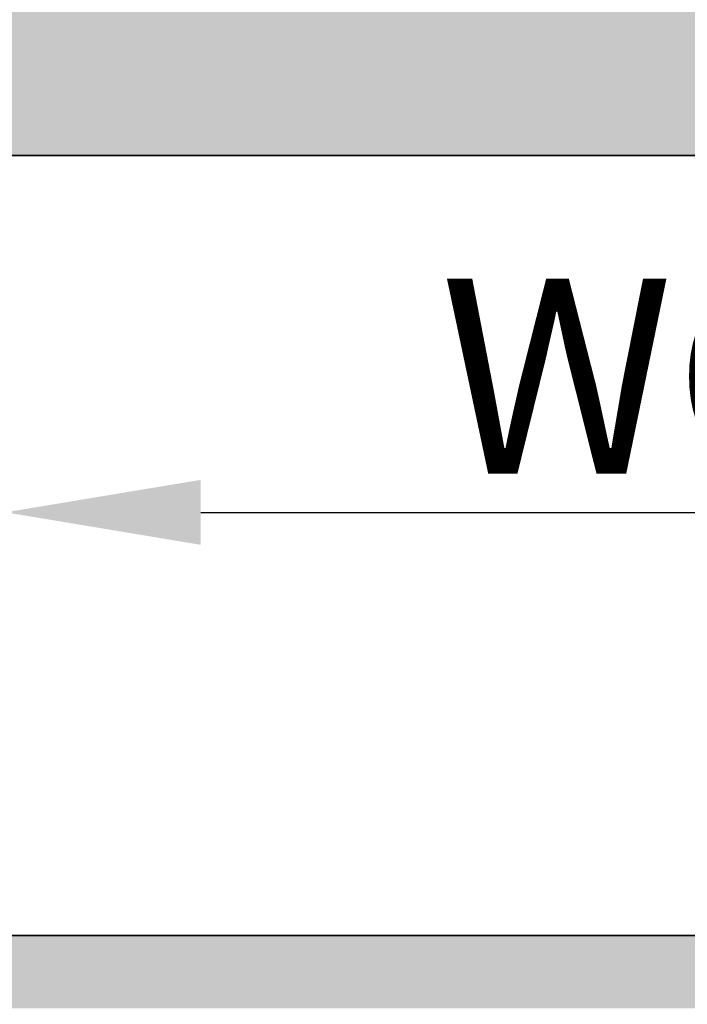
# Model space of a CAD drawing. Units: inches. Extents: x 2083 to 3317, y 1141 to 2115.
# Tile 17 of 256: x 2255 to 2296, y 1417 to 1477. Entities that reach past the tile are written whole.
import ezdxf

# ---------------------------------------------------------------- set-up
doc = ezdxf.new("R2010")
doc.units = ezdxf.units.IN
doc.layers.add('A-ANNO-DIMS', color=2, linetype='Continuous', lineweight=18)
doc.layers.add('A-WALL', color=7, linetype='Continuous', lineweight=35)
doc.layers.add('A-WALL-PATT', color=251, linetype='Continuous', lineweight=13, true_color=0x636466)
doc.styles.get("Standard").update_dxf_attribs({"font": 'arial.ttf'})
doc.dimstyles.new('ISO-25', dxfattribs={"dimtxt": 12, "dimasz": 12, "dimexe": 1.25, "dimexo": 0.625, "dimtad": 1, "dimlunit": 3, "dimtxsty": 'Standard', "dimcen": 2.5, "dimadec": 0, "dimazin": 0, "dimtfac": 1, "dimtmove": 0, "dimatfit": 3, "dimfxl": 1, "dimarcsym": 0})

# ---------------------------------------------------------------- blocks, each defined once
blk = doc.blocks.new('*D22')
at = {"layer": 'A-ANNO-DIMS', "color": 0, "lineweight": -2, "transparency": 16777216}
for p, q in [((2235.96, 1362.739), (2235.96, 1376.309)), ((2322.26, 1362.739), (2322.26, 1376.309)), ((2235.96, 1375.059), (2083.007, 1375.059)), ((2310.26, 1375.059), (2247.96, 1375.059))]:
    blk.add_line(p, q, dxfattribs=at)
at = {"layer": 'A-ANNO-DIMS', "color": 0, "transparency": 16777216}
for points in [[(2247.96, 1377.059), (2247.96, 1373.059), (2235.96, 1375.059)], [(2310.26, 1377.059), (2310.26, 1373.059), (2322.26, 1375.059)]]:
    blk.add_solid(points, dxfattribs=at)
at = {"layer": 'Defpoints', "color": 0, "transparency": 16777216}
for p in [(2235.96, 1375.059), (2235.96, 1362.114), (2322.26, 1362.114)]:
    blk.add_point(p, dxfattribs=at)
at = {"layer": 'A-ANNO-DIMS', "color": 0, "transparency": 16777216, "insert": (2153.483, 1381.889), "char_height": 12, "attachment_point": 5}
blk.add_mtext('BED 7\'-2 1/2" TYP.', dxfattribs=at)
blk = doc.blocks.new('*D30')
at = {"layer": 'A-ANNO-DIMS', "color": 0, "lineweight": -2, "transparency": 16777216}
for p, q in [((2240.018, 1445.274), (2240.018, 1448.046)), ((2254.329, 1445.274), (2254.329, 1448.046)), ((2228.018, 1446.796), (2216.018, 1446.796)), ((2240.018, 1446.796), (2254.329, 1446.796)), ((2266.329, 1446.796), (2413.765, 1446.796))]:
    blk.add_line(p, q, dxfattribs=at)
at = {"layer": 'A-ANNO-DIMS', "color": 0, "transparency": 16777216}
for points in [[(2228.018, 1448.796), (2228.018, 1444.796), (2240.018, 1446.796)], [(2266.329, 1448.796), (2266.329, 1444.796), (2254.329, 1446.796)]]:
    blk.add_solid(points, dxfattribs=at)
at = {"layer": 'Defpoints', "color": 0, "transparency": 16777216}
for p in [(2254.329, 1446.796), (2240.018, 1444.649), (2254.329, 1444.649)]:
    blk.add_point(p, dxfattribs=at)
at = {"layer": 'A-ANNO-DIMS', "color": 0, "transparency": 16777216, "insert": (2346.047, 1453.625), "char_height": 12, "attachment_point": 5}
blk.add_mtext('WC 1\'-2 1/2" TYP.', dxfattribs=at)
blk = doc.blocks.new('*D62')
at = {"layer": 'A-ANNO-DIMS', "color": 0, "lineweight": -2, "transparency": 16777216}
for p, q in [((2235.96, 1469.386), (2235.96, 1522.361)), ((2379.96, 1469.386), (2379.96, 1522.361)), ((2247.96, 1521.111), (2367.96, 1521.111))]:
    blk.add_line(p, q, dxfattribs=at)
at = {"layer": 'A-ANNO-DIMS', "color": 0, "transparency": 16777216}
for points in [[(2247.96, 1523.111), (2247.96, 1519.111), (2235.96, 1521.111)], [(2367.96, 1523.111), (2367.96, 1519.111), (2379.96, 1521.111)]]:
    blk.add_solid(points, dxfattribs=at)
at = {"layer": 'Defpoints', "color": 0, "transparency": 16777216}
for p in [(2379.96, 1521.111), (2235.96, 1468.761), (2379.96, 1468.761)]:
    blk.add_point(p, dxfattribs=at)
at = {"layer": 'A-ANNO-DIMS', "color": 0, "transparency": 16777216, "insert": (2307.96, 1527.863), "char_height": 12, "attachment_point": 5}
blk.add_mtext('12\'-0"', dxfattribs=at)

msp = doc.modelspace()

# ---------------------------------------------------------------- hatches: boundary and pattern name
at = {"layer": 'A-WALL-PATT'}
h = msp.add_hatch(color=256, dxfattribs=at)
h.dxf.hatch_style = 1
h.paths.add_polyline_path([(3126.96, 2020.761), (2748.96, 2020.761), (2604.96, 2020.761), (2226.96, 2020.761), (2226.96, 1702.761), (2466.96, 1702.761), (2466.96, 1582.761), (2418.96, 1582.761), (2418.96, 1477.761), (2226.96, 1477.761), (2226.96, 1263.261), (2544.96, 1263.261), (2544.96, 1411.761), (2604.96, 1411.761), (2685.96, 1411.761), (2685.96, 1420.761), (2604.96, 1420.761), (2604.96, 1573.761), (2604.96, 1702.761), (2604.96, 2011.761), (2748.96, 2011.761), (2748.96, 1702.761), (2862.96, 1702.761), (2862.96, 1621.761), (2871.96, 1621.761), (2871.96, 1702.761), (2883.96, 1702.761), (2883.96, 1706.939, -0.026459), (2883.96, 1711.761), (2757.96, 1711.761), (2757.96, 1807.761), (2787.96, 1807.761), (2787.96, 1812.261), (2757.96, 1812.261), (2757.96, 2011.761), (2877.96, 2011.761), (2877.96, 1812.261), (2847.96, 1812.261), (2847.96, 1807.761), (2889.836, 1807.761), (2889.836, 1812.261), (2882.46, 1812.261), (2882.46, 2011.761), (3117.96, 2011.761), (3117.96, 1812.261), (2937.836, 1812.261), (2937.836, 1807.761), (2995.71, 1807.761), (2995.71, 1796.118), (3000.21, 1796.118), (3000.21, 1807.761), (3117.96, 1807.761), (3117.96, 1711.761), (3000.21, 1711.761), (3000.21, 1760.118), (2998.573, 1760.118, -0.020711), (2995.71, 1760.118), (2995.71, 1711.761), (2931.96, 1711.761), (2931.96, 1702.761), (3126.96, 1702.761)])
h.paths.add_polyline_path([(2471.46, 2011.761), (2471.46, 1810.011), (2462.717, 1810.011), (2462.717, 1805.511), (2505.96, 1805.511), (2505.96, 1810.011), (2475.96, 1810.011), (2475.96, 2011.761), (2595.96, 2011.761), (2595.96, 1810.011), (2565.96, 1810.011), (2565.96, 1805.511), (2595.96, 1805.511), (2595.96, 1711.761), (2235.96, 1711.761), (2235.96, 1805.511), (2353.71, 1805.511), (2353.71, 1796.054), (2358.21, 1796.054), (2358.21, 1805.511), (2414.717, 1805.511), (2414.717, 1810.011), (2235.96, 1810.011), (2235.96, 2011.761)], flags=16)
h.paths.add_polyline_path([(2270.205, 1994.61), (2270.205, 1970.61), (2246.205, 1970.61), (2246.205, 1994.61)], flags=0)
edge = h.paths.add_edge_path(flags=0)
edge.add_ellipse((2332.027, 1899.798), major_axis=(-3.043, 3.043), ratio=0.168252, start_angle=-161.33217, end_angle=-156.30711, ccw=False)
edge.add_ellipse((2333.082, 1898.744), major_axis=(-1.055, 1.055), ratio=0.453532, start_angle=-123.37102, end_angle=-94.15911)
edge = h.paths.add_edge_path(flags=0)
edge.add_ellipse((2332.027, 1968.876), major_axis=(3.043, 3.043), ratio=0.168252, start_angle=18.66783, end_angle=23.69289)
edge.add_spline(control_points=[(2332.926, 1970.691), (2332.227, 1970.336), (2330.894, 1969.659), (2328.413, 1970.932), (2327.204, 1967.749), (2324.71, 1969.956), (2322.533, 1967.012), (2320.013, 1971.296), (2317.68, 1968.158), (2316.041, 1967.102), (2315.427, 1966.81)], knot_values=[0, 0, 0, 0, 2.267059, 4.324559, 6.685584, 8.878641, 11.121502, 14.300359, 17.755284, 19.732645, 19.732645, 19.732645, 19.732645], degree=3, periodic=0)
edge.add_ellipse((2332.027, 1968.876), major_axis=(3.043, 3.043), ratio=0.168252, start_angle=18.66783, end_angle=23.69289, ccw=False)
edge.add_ellipse((2333.082, 1969.931), major_axis=(1.055, 1.055), ratio=0.453532, start_angle=56.62898, end_angle=85.84089, ccw=False)
edge = h.paths.add_edge_path(flags=0)
edge.add_spline(control_points=[(2296.428, 1967.988), (2293.628, 1965.336), (2287.704, 1959.727), (2299.744, 1949.996), (2294.533, 1935.669), (2290.573, 1920.604), (2293.394, 1909.974), (2296.185, 1904.967)], knot_values=[0.099185, 0.099185, 0.099185, 0.099185, 0.345301, 0.619822, 0.982653, 1.386093, 1.810555, 1.810555, 1.810555, 1.810555], degree=3, periodic=0)
edge.add_spline(control_points=[(2296.185, 1904.967), (2297.384, 1902.619), (2298.001, 1901.949), (2298.553, 1901.468)], knot_values=[0.006246, 0.006246, 0.006246, 0.006246, 0.055476, 0.055476, 0.055476, 0.055476], degree=3, periodic=0)
edge.add_spline(control_points=[(2298.553, 1901.468), (2297.259, 1900.923), (2295.225, 1900.232), (2293.06, 1900.614), (2292.101, 1900.788), (2292.09, 1900.791)], knot_values=[0.312835, 0.312835, 0.312835, 0.312835, 0.40178, 0.474987, 0.475903, 0.475903, 0.475903, 0.475903], degree=3, periodic=0)
edge.add_arc((2292.794, 1904.664), 3.937, 215.4209, 259.69818, ccw=False)
edge.add_spline(control_points=[(2289.585, 1902.382), (2289.477, 1902.535), (2289.368, 1902.688), (2289.261, 1902.841)], knot_values=[0.102872, 0.102872, 0.102872, 0.102872, 0.116896, 0.116896, 0.116896, 0.116896], degree=3, periodic=0)
edge.add_spline(control_points=[(2289.261, 1902.841), (2288.687, 1902.55), (2287.64, 1902.02), (2285.881, 1901.874), (2283.853, 1901.504), (2281.72, 1899.711), (2278.467, 1899.493), (2276.157, 1901.883), (2272.259, 1899.804), (2267.778, 1901.843), (2262.244, 1900.184), (2257.415, 1901.782), (2254.318, 1900.726), (2253.178, 1900.337)], knot_values=[0, 0, 0, 0, 1.907977, 3.477176, 5.261074, 7.972851, 11.680248, 13.717921, 16.939592, 22.789562, 27.502503, 33.595215, 37.145618, 37.145618, 37.145618, 37.145618], degree=3, periodic=0)
edge.add_line((2253.178, 1900.337), (2250.244, 1902.841))
edge.add_line((2250.244, 1902.841), (2250.244, 1965.833))
edge.add_line((2250.244, 1965.833), (2253.178, 1968.337))
edge.add_spline(control_points=[(2253.178, 1968.337), (2254.318, 1967.948), (2257.415, 1966.892), (2262.244, 1968.49), (2267.778, 1966.831), (2271.527, 1968.537), (2273.876, 1967.828), (2274.207, 1967.728)], knot_values=[0, 0, 0, 0, 0.09018, 0.244935, 0.364644, 0.513233, 0.537855, 0.537855, 0.537855, 0.537855], degree=3, periodic=0)
edge.add_arc((2274.353, 1963.793), 3.937, 72.05113, 92.12795, ccw=False)
edge.add_arc((2281.297, 1985.23), 18.596, 252.05113, 288.56572)
edge.add_arc((2292.317, 1956.029), 12.646, 71.02679, 113.77822, ccw=False)
edge = h.paths.add_edge_path(flags=0)
edge.add_spline(control_points=[(2274.899, 1951.856), (2275.066, 1951.617), (2275.233, 1951.377), (2275.398, 1951.136)], knot_values=[1.409916, 1.409916, 1.409916, 1.409916, 1.43159, 1.43159, 1.43159, 1.43159], degree=3, periodic=0)
edge.add_spline(control_points=[(2275.398, 1951.136), (2275.792, 1950.562), (2276.179, 1949.984), (2276.546, 1949.397)], knot_values=[1.358238, 1.358238, 1.358238, 1.358238, 1.409916, 1.409916, 1.409916, 1.409916], degree=3, periodic=0)
edge.add_line((2276.546, 1949.397), (2277.437, 1947.862))
edge.add_spline(control_points=[(2277.437, 1947.862), (2276.304, 1945.673), (2274.64, 1942.427), (2274.632, 1938.094), (2272.799, 1930.852), (2274.356, 1943.897), (2275.948, 1947.923), (2276.546, 1949.397)], knot_values=[0.005632, 0.005632, 0.005632, 0.005632, 0.186014, 0.266002, 0.357087, 0.59639, 0.739732, 0.739732, 0.739732, 0.739732], degree=3, periodic=0)
edge.add_spline(control_points=[(2276.546, 1949.397), (2276.179, 1949.984), (2275.792, 1950.562), (2275.398, 1951.136)], knot_values=[1.358238, 1.358238, 1.358238, 1.358238, 1.409916, 1.409916, 1.409916, 1.409916], degree=3, periodic=0)
edge.add_spline(control_points=[(2275.398, 1951.136), (2274.943, 1950.08), (2274.208, 1948.025), (2273.935, 1944.851), (2272.469, 1937.627), (2273.466, 1945.696), (2274.701, 1951.059), (2274.899, 1951.856)], knot_values=[0.104364, 0.104364, 0.104364, 0.104364, 0.189636, 0.269624, 0.36071, 0.600013, 0.644622, 0.644622, 0.644622, 0.644622], degree=3, periodic=0)
h.paths.add_polyline_path([(2269.168, 1963.128, -0.357527), (2268.171, 1960.976, -0.092561), (2268.171, 1939.436, -0.357527), (2269.168, 1937.285, -0.357527), (2267.016, 1938.282, -0.164785), (2254.686, 1938.282, -0.357527), (2252.534, 1937.285, -0.357527), (2253.531, 1939.436, -0.092561), (2253.531, 1960.976, -0.357527), (2252.534, 1963.128, -0.357527), (2254.686, 1962.131, -0.164785), (2267.016, 1962.131, -0.357527)], flags=0)
h.paths.add_polyline_path([(2248.874, 1967.802), (2248.874, 1957.028), (2249.458, 1957.028), (2249.458, 1911.647), (2248.874, 1911.647), (2248.874, 1900.873), (2246.512, 1900.873, 0.197327), (2244.15, 1902.457), (2244.15, 1966.218, 0.197327), (2246.512, 1967.802)], flags=0)
h.paths.add_polyline_path([(2269.168, 1931.389, -0.357527), (2268.171, 1929.238, -0.092561), (2268.171, 1907.698, -0.357527), (2269.168, 1905.547, -0.357527), (2267.016, 1906.544, -0.164785), (2254.686, 1906.544, -0.357527), (2252.534, 1905.547, -0.357527), (2253.531, 1907.698, -0.092561), (2253.531, 1929.238, -0.357527), (2252.534, 1931.389, -0.357527), (2254.686, 1930.392, -0.164785), (2267.016, 1930.392, -0.357527)], flags=0)
edge = h.paths.add_edge_path(flags=0)
edge.add_spline(control_points=[(2276.197, 1906.724), (2276.168, 1909.029), (2276.114, 1913.372), (2270.598, 1924.925), (2273.905, 1919.013), (2275.922, 1916.262), (2275.475, 1912.402), (2277.258, 1910.381), (2276.696, 1908.225), (2276.646, 1906.813), (2276.618, 1906.008)], knot_values=[0, 0, 0, 0, 8.61026, 16.221274, 18.843057, 23.804898, 27.440828, 29.356102, 31.203478, 33.650687, 33.650687, 33.650687, 33.650687], degree=3, periodic=0)
edge.add_spline(control_points=[(2276.618, 1906.008), (2276.623, 1905.624), (2276.498, 1904.629), (2275.442, 1903.855), (2274.937, 1903.08), (2274.859, 1902.841)], knot_values=[0.156488, 0.156488, 0.156488, 0.156488, 0.184398, 0.231376, 0.250598, 0.250598, 0.250598, 0.250598], degree=3, periodic=0)
edge.add_line((2274.859, 1902.841), (2276.506, 1902.841))
edge.add_spline(control_points=[(2276.506, 1902.841), (2276.788, 1903.085), (2277.665, 1904.125), (2278.25, 1904.341), (2277.654, 1908.527), (2278.156, 1906.228), (2278.1, 1905.286), (2278.847, 1904.069), (2277.857, 1903.415), (2277.874, 1902.991), (2277.904, 1902.841)], knot_values=[0.059574, 0.059574, 0.059574, 0.059574, 0.080753, 0.103741, 0.16972, 0.176036, 0.207137, 0.240474, 0.262341, 0.27366, 0.27366, 0.27366, 0.27366], degree=3, periodic=0)
edge.add_line((2277.904, 1902.841), (2280.03, 1902.841))
edge.add_spline(control_points=[(2280.03, 1902.841), (2279.888, 1903.088), (2279.499, 1903.982), (2280.152, 1905.939), (2278.104, 1909.658), (2279.762, 1907.185), (2280.328, 1904.875), (2280.485, 1903.49), (2281.463, 1903.249), (2281.758, 1902.936), (2281.834, 1902.841)], knot_values=[0.013856, 0.013856, 0.013856, 0.013856, 0.034874, 0.088867, 0.107879, 0.126738, 0.158714, 0.193757, 0.217487, 0.226722, 0.226722, 0.226722, 0.226722], degree=3, periodic=0)
edge.add_spline(control_points=[(2281.834, 1902.841), (2281.788, 1902.827), (2281.647, 1902.783), (2281.396, 1902.859), (2281.088, 1902.985), (2280.721, 1903.061), (2280.333, 1903.026), (2280.125, 1902.899), (2280.03, 1902.841)], knot_values=[0, 0, 0, 0, 0.14413, 0.435517, 0.749276, 1.153046, 1.548371, 1.878348, 1.878348, 1.878348, 1.878348], degree=3, periodic=0)
edge.add_line((2280.03, 1902.841), (2277.904, 1902.841))
edge.add_spline(control_points=[(2277.904, 1902.841), (2277.893, 1902.796), (2277.865, 1902.68), (2277.607, 1902.687), (2277.274, 1902.801), (2276.838, 1902.62), (2276.584, 1902.789), (2276.506, 1902.841)], knot_values=[0, 0, 0, 0, 0.127189, 0.326199, 0.628009, 1.24357, 1.515331, 1.515331, 1.515331, 1.515331], degree=3, periodic=0)
edge.add_line((2276.506, 1902.841), (2274.859, 1902.841))
edge.add_spline(control_points=[(2274.859, 1902.841), (2274.814, 1902.899), (2274.725, 1903.013), (2274.493, 1903.119), (2274.244, 1902.961), (2273.937, 1903.185), (2273.614, 1902.983), (2273.408, 1902.883), (2273.322, 1902.841)], knot_values=[0, 0, 0, 0, 0.21843, 0.436957, 0.687977, 0.990379, 1.398396, 1.69185, 1.69185, 1.69185, 1.69185], degree=3, periodic=0)
edge.add_spline(control_points=[(2273.322, 1902.841), (2273.617, 1903.446), (2274.274, 1904.538), (2276.027, 1904.574), (2276.207, 1906.584), (2276.197, 1906.724)], knot_values=[0.012227, 0.012227, 0.012227, 0.012227, 0.059472, 0.106218, 0.134458, 0.134458, 0.134458, 0.134458], degree=3, periodic=0)
h.paths.add_polyline_path([(2270.776, 1897.79), (2270.776, 1873.79), (2246.776, 1873.79), (2246.776, 1897.79)], flags=0)
h.paths.add_polyline_path([(2353.71, 1760.005), (2353.71, 1760.054), (2358.21, 1760.054, -0.033729)], flags=0)
h.paths.add_polyline_path([(2321.819, 1737.529), (2341.995, 1737.529, -0.414214), (2343.203, 1736.321), (2343.203, 1721.021, -0.414214), (2341.995, 1719.813), (2321.819, 1719.813, -0.414214), (2320.611, 1721.021), (2320.611, 1736.321, -0.414214)], flags=0)
h.paths.add_polyline_path([(2324.235, 1736.321), (2339.579, 1736.321, -0.414214), (2341.995, 1733.905), (2341.995, 1725.45, -0.414214), (2339.579, 1723.034), (2333.681, 1723.034), (2333.845, 1722.045, -0.870646), (2335.425, 1721.826, -0.767327), (2333.923, 1721.423), (2331.291, 1721.423, -0.767327), (2329.788, 1721.826, -0.870646), (2331.368, 1722.045), (2331.533, 1723.034), (2324.235, 1723.034, -0.414214), (2321.819, 1725.45), (2321.819, 1733.905, -0.414214)], flags=0)
h.paths.add_polyline_path([(2570.484, 1928.615), (2589.684, 1928.615), (2590.169, 1928.615), (2590.169, 1904.993), (2570.484, 1904.993)], flags=0)
h.paths.add_polyline_path([(2574.447, 1927.264, -1), (2572.829, 1927.264, -1)], flags=0)
h.paths.add_polyline_path([(2573.09, 1926.941), (2573.925, 1927.776), (2574.148, 1927.553), (2573.313, 1926.718)], flags=0)
h.paths.add_polyline_path([(2578.779, 1919.73, -1), (2571.592, 1919.73, -1)], flags=0)
h.paths.add_polyline_path([(2578.385, 1919.73, -1), (2571.985, 1919.73, -1)], flags=0)
h.paths.add_polyline_path([(2331.596, 1729.476, -1), (2333.618, 1729.476, -1)], flags=0)
h.paths.add_polyline_path([(2578.034, 1927.264, -1), (2576.416, 1927.264, -1)], flags=0)
h.paths.add_polyline_path([(2576.689, 1927.531), (2576.912, 1927.754), (2577.747, 1926.919), (2577.524, 1926.696)], flags=0)
h.paths.add_polyline_path([(2578.139, 1909.86, -1), (2572.232, 1909.86, -1)], flags=0)
h.paths.add_polyline_path([(2577.745, 1909.86, -1), (2572.625, 1909.86, -1)], flags=0)
h.paths.add_polyline_path([(2583.798, 1927.264, -1), (2582.179, 1927.264, -1)], flags=0)
h.paths.add_polyline_path([(2582.719, 1927.754), (2583.554, 1926.919), (2583.331, 1926.696), (2582.496, 1927.531)], flags=0)
h.paths.add_polyline_path([(2582.496, 1927.531), (2582.719, 1927.754), (2583.554, 1926.919), (2583.331, 1926.696)], flags=0)
h.paths.add_polyline_path([(2587.739, 1920.53, -1), (2581.832, 1920.53, -1)], flags=0)
h.paths.add_polyline_path([(2587.345, 1920.53, -1), (2582.225, 1920.53, -1)], flags=0)
h.paths.add_polyline_path([(2587.385, 1927.264, -1), (2585.766, 1927.264, -1)], flags=0)
h.paths.add_polyline_path([(2586.082, 1926.98), (2586.917, 1927.815), (2587.14, 1927.593), (2586.305, 1926.758)], flags=0)
h.paths.add_polyline_path([(2588.379, 1910.66, -1), (2581.192, 1910.66, -1)], flags=0)
h.paths.add_polyline_path([(2587.985, 1910.66, -1), (2581.585, 1910.66, -1)], flags=0)
h.paths.add_polyline_path([(2417.168, 1729.478), (2437.344, 1729.478, -0.414214), (2438.552, 1728.27), (2438.552, 1712.969, -0.414214), (2437.344, 1711.761), (2417.168, 1711.761, -0.414214), (2415.96, 1712.969), (2415.96, 1728.27, -0.414214)], flags=0)
h.paths.add_polyline_path([(2419.584, 1728.27), (2434.928, 1728.27, -0.414214), (2437.344, 1725.854), (2437.344, 1717.398, -0.414214), (2434.928, 1714.983), (2429.029, 1714.983), (2429.194, 1713.994, -0.870646), (2430.774, 1713.775, -0.767327), (2429.271, 1713.372), (2426.64, 1713.372, -0.767327), (2425.137, 1713.775, -0.870646), (2426.717, 1713.994), (2426.882, 1714.983), (2419.584, 1714.983, -0.414214), (2417.168, 1717.398), (2417.168, 1725.854, -0.414214)], flags=0)
h.paths.add_polyline_path([(2419.584, 1728.27), (2434.928, 1728.27, -0.414214), (2437.344, 1725.854), (2437.344, 1717.398, -0.414214), (2434.928, 1714.983), (2429.029, 1714.983), (2428.358, 1719.009), (2427.553, 1719.009), (2426.882, 1714.983), (2419.584, 1714.983, -0.414214), (2417.168, 1717.398), (2417.168, 1725.854, -0.414214)], flags=0)
h.paths.add_polyline_path([(2426.944, 1721.425, -1), (2428.967, 1721.425, -1)], flags=0)
h.paths.add_polyline_path([(2475.96, 1702.761), (2595.96, 1702.761), (2595.96, 1582.761), (2475.96, 1582.761)], flags=16)
h.paths.add_polyline_path([(2427.96, 1573.761), (2595.96, 1573.761), (2595.96, 1468.761), (2595.96, 1420.761), (2384.46, 1420.761), (2384.46, 1468.761), (2427.96, 1468.761)], flags=16)
h.paths.add_polyline_path([(2379.96, 1468.761), (2379.96, 1420.761), (2235.96, 1420.761), (2235.96, 1468.761)], flags=16)
h.paths.add_polyline_path([(2317.816, 1466.696), (2337.992, 1466.696, -0.414214), (2339.2, 1465.488), (2339.2, 1450.187, -0.414214), (2337.992, 1448.979), (2317.816, 1448.979, -0.414214), (2316.608, 1450.187), (2316.608, 1465.488, -0.414214)], flags=0)
h.paths.add_polyline_path([(2320.232, 1465.488), (2335.576, 1465.488, -0.414214), (2337.992, 1463.072), (2337.992, 1454.616, -0.414214), (2335.576, 1452.2), (2329.677, 1452.2), (2329.842, 1451.212, -0.870646), (2331.422, 1450.992, -0.767327), (2329.92, 1450.59), (2327.288, 1450.59, -0.767327), (2325.785, 1450.992, -0.870646), (2327.365, 1451.212), (2327.53, 1452.2), (2320.232, 1452.2, -0.414214), (2317.816, 1454.616), (2317.816, 1463.072, -0.414214)], flags=0)
h.paths.add_polyline_path([(2320.232, 1465.488), (2335.576, 1465.488, -0.414214), (2337.992, 1463.072), (2337.992, 1454.616, -0.414214), (2335.576, 1452.2), (2329.677, 1452.2), (2329.006, 1456.227), (2328.201, 1456.227), (2327.53, 1452.2), (2320.232, 1452.2, -0.414214), (2317.816, 1454.616), (2317.816, 1463.072, -0.414214)], flags=0)
h.paths.add_polyline_path([(2327.593, 1458.643, -1), (2329.615, 1458.643, -1)], flags=0)
h.paths.add_polyline_path([(2244.412, 1433.34), (2241.921, 1433.34, -0.414214), (2240.018, 1435.244), (2240.018, 1440.953, -0.414211), (2241.921, 1442.856), (2244.412, 1442.856, -1.976472)], flags=0)
h.paths.add_polyline_path([(2245.357, 1434.398, -0.414214), (2245.357, 1441.799, -2.144098)], flags=0)
h.paths.add_polyline_path([(2535.96, 1416.261), (2535.96, 1272.261), (2235.96, 1272.261), (2235.96, 1416.261)], flags=16)
h.paths.add_polyline_path([(2260.12, 1384.293), (2260.12, 1362.039), (2237.865, 1362.039), (2237.865, 1384.293)], flags=0)
edge = h.paths.add_edge_path(flags=0)
edge.add_line((2318.252, 1362.093), (2318.146, 1362.001))
edge.add_ellipse((2317.445, 1360.431), major_axis=(2.822, 2.822), ratio=0.168252, start_angle=18.66783, end_angle=20.94813, ccw=False)
edge.add_ellipse((2318.423, 1361.409), major_axis=(0.978, 0.978), ratio=0.453532, start_angle=56.62898, end_angle=70.2262, ccw=False)
edge = h.paths.add_edge_path(flags=0)
edge.add_line((2319.107, 1295.571), (2319.015, 1295.677))
edge.add_ellipse((2317.445, 1296.378), major_axis=(-2.822, 2.822), ratio=0.168252, start_angle=-161.33217, end_angle=-159.05187, ccw=False)
edge.add_ellipse((2318.423, 1295.4), major_axis=(-0.978, 0.978), ratio=0.453532, start_angle=-123.37102, end_angle=-109.7738)
edge = h.paths.add_edge_path(flags=0)
edge.add_spline(control_points=[(2284.21, 1301.17), (2284.581, 1300.445), (2284.891, 1299.892), (2285.16, 1299.461)], knot_values=[0.039066, 0.039066, 0.039066, 0.039066, 0.055476, 0.055476, 0.055476, 0.055476], degree=3, periodic=0)
edge.add_line((2285.16, 1299.461), (2284.21, 1301.17))
edge = h.paths.add_edge_path(flags=0)
edge.add_line((2280.412, 1297.298), (2283.37, 1297.036))
edge.add_line((2283.37, 1297.036), (2286.406, 1297.926))
edge.add_spline(control_points=[(2286.406, 1297.926), (2285.305, 1297.463), (2284.345, 1297.129), (2283.37, 1297.036)], knot_values=[0.394369, 0.394369, 0.394369, 0.394369, 0.475903, 0.475903, 0.475903, 0.475903], degree=3, periodic=0)
edge.add_spline(control_points=[(2283.37, 1297.036), (2283.281, 1297.028), (2282.316, 1296.957), (2281.313, 1297.134), (2280.423, 1297.296), (2280.412, 1297.298)], knot_values=[0.312835, 0.312835, 0.312835, 0.312835, 0.320246, 0.393453, 0.394369, 0.394369, 0.394369, 0.394369], degree=3, periodic=0)
edge = h.paths.add_edge_path(flags=0)
edge.add_line((2284.436, 1359.607), (2280.446, 1355.328))
edge.add_line((2280.446, 1355.328), (2279.58, 1351.018))
edge.add_line((2279.58, 1351.018), (2282.413, 1346.58))
edge.add_spline(control_points=[(2282.413, 1346.58), (2283.153, 1345.589), (2284.253, 1344.029), (2284.801, 1342.387), (2284.935, 1341.806)], knot_values=[1.240098, 1.240098, 1.240098, 1.240098, 1.332892, 1.382712, 1.382712, 1.382712, 1.382712], degree=3, periodic=0)
edge.add_spline(control_points=[(2284.935, 1341.806), (2285.319, 1340.141), (2285.233, 1338.409), (2284.91, 1336.654)], knot_values=[1.097484, 1.097484, 1.097484, 1.097484, 1.240098, 1.240098, 1.240098, 1.240098], degree=3, periodic=0)
edge.add_spline(control_points=[(2284.91, 1336.654), (2284.587, 1334.899), (2284.027, 1333.12), (2283.463, 1331.361)], knot_values=[0.95487, 0.95487, 0.95487, 0.95487, 1.097484, 1.097484, 1.097484, 1.097484], degree=3, periodic=0)
edge.add_line((2283.463, 1331.361), (2281.89, 1326.153))
edge.add_line((2281.89, 1326.153), (2280.756, 1321.056))
edge.add_line((2280.756, 1321.056), (2280.299, 1316.002))
edge.add_line((2280.299, 1316.002), (2280.716, 1310.95))
edge.add_line((2280.716, 1310.95), (2282.028, 1305.972))
edge.add_line((2282.028, 1305.972), (2284.21, 1301.17))
edge.add_spline(control_points=[(2284.21, 1301.17), (2283.341, 1302.73), (2282.612, 1304.336), (2282.028, 1305.972)], knot_values=[0.099185, 0.099185, 0.099185, 0.099185, 0.241799, 0.241799, 0.241799, 0.241799], degree=3, periodic=0)
edge.add_spline(control_points=[(2282.028, 1305.972), (2281.444, 1307.608), (2281.005, 1309.273), (2280.716, 1310.95)], knot_values=[0.241799, 0.241799, 0.241799, 0.241799, 0.384413, 0.384413, 0.384413, 0.384413], degree=3, periodic=0)
edge.add_spline(control_points=[(2280.716, 1310.95), (2280.433, 1312.588), (2280.289, 1314.277), (2280.299, 1315.962), (2280.299, 1316.002)], knot_values=[0.384413, 0.384413, 0.384413, 0.384413, 0.523647, 0.527028, 0.527028, 0.527028, 0.527028], degree=3, periodic=0)
edge.add_spline(control_points=[(2280.299, 1316.002), (2280.312, 1317.687), (2280.478, 1319.368), (2280.756, 1321.056)], knot_values=[0.527028, 0.527028, 0.527028, 0.527028, 0.669642, 0.669642, 0.669642, 0.669642], degree=3, periodic=0)
edge.add_spline(control_points=[(2280.756, 1321.056), (2281.035, 1322.744), (2281.426, 1324.44), (2281.89, 1326.153)], knot_values=[0.669642, 0.669642, 0.669642, 0.669642, 0.812256, 0.812256, 0.812256, 0.812256], degree=3, periodic=0)
edge.add_spline(control_points=[(2281.89, 1326.153), (2282.264, 1327.533), (2282.788, 1329.262), (2283.353, 1331.018), (2283.463, 1331.361)], knot_values=[0.812256, 0.812256, 0.812256, 0.812256, 0.927087, 0.95487, 0.95487, 0.95487, 0.95487], degree=3, periodic=0)
edge.add_line((2283.463, 1331.361), (2284.91, 1336.654))
edge.add_line((2284.91, 1336.654), (2284.935, 1341.806))
edge.add_line((2284.935, 1341.806), (2282.413, 1346.58))
edge.add_spline(control_points=[(2282.413, 1346.58), (2281.275, 1348.104), (2280.078, 1349.57), (2279.58, 1351.018)], knot_values=[1.382712, 1.382712, 1.382712, 1.382712, 1.525326, 1.525326, 1.525326, 1.525326], degree=3, periodic=0)
edge.add_spline(control_points=[(2279.58, 1351.018), (2279.443, 1351.415), (2279.136, 1352.857), (2279.735, 1354.29), (2280.446, 1355.328)], knot_values=[1.525326, 1.525326, 1.525326, 1.525326, 1.564439, 1.667941, 1.667941, 1.667941, 1.667941], degree=3, periodic=0)
edge.add_spline(control_points=[(2280.446, 1355.328), (2281.426, 1356.758), (2282.931, 1358.183), (2284.436, 1359.607)], knot_values=[1.667941, 1.667941, 1.667941, 1.667941, 1.810555, 1.810555, 1.810555, 1.810555], degree=3, periodic=0)
edge.add_arc((2280.623, 1348.518), 11.726, 71.02679, 113.77822)
edge.add_arc((2270.405, 1375.595), 17.244, 252.05113, 288.56572, ccw=False)
edge.add_arc((2263.966, 1355.718), 3.651, 72.05113, 92.12795)
edge.add_arc((2263.966, 1355.718), 3.651, 92.12795, 177.98513)
edge.add_spline(control_points=[(2260.318, 1355.846), (2260.26, 1354.221), (2260.551, 1350.187), (2262.999, 1346.766), (2264.473, 1344.649)], knot_values=[1.43159, 1.43159, 1.43159, 1.43159, 1.564144, 1.770695, 1.770695, 1.770695, 1.770695], degree=3, periodic=0)
edge.add_line((2264.473, 1344.649), (2264.936, 1343.983))
edge.add_spline(control_points=[(2263.801, 1340.248), (2263.843, 1340.514), (2264.067, 1341.756), (2264.513, 1343.002), (2264.935, 1343.981)], knot_values=[0.53657, 0.53657, 0.53657, 0.53657, 0.559349, 0.644622, 0.644622, 0.644622, 0.644622], degree=3, periodic=0)
edge.add_spline(control_points=[(2264.935, 1343.981), (2265.118, 1343.715), (2265.299, 1343.448), (2265.477, 1343.179)], knot_values=[1.384077, 1.384077, 1.384077, 1.384077, 1.409916, 1.409916, 1.409916, 1.409916], degree=3, periodic=0)
edge.add_spline(control_points=[(2265.477, 1343.179), (2265.655, 1342.911), (2265.829, 1342.641), (2265.999, 1342.369)], knot_values=[1.358238, 1.358238, 1.358238, 1.358238, 1.384077, 1.384077, 1.384077, 1.384077], degree=3, periodic=0)
edge.add_line((2265.999, 1342.369), (2266.826, 1340.946))
edge.add_spline(control_points=[(2266.826, 1340.946), (2268.894, 1337.09), (2271.398, 1325.843), (2270.516, 1310.569), (2275.919, 1301.861), (2277.79, 1299.199)], knot_values=[0.116896, 0.116896, 0.116896, 0.116896, 0.472987, 1.050969, 1.313793, 1.313793, 1.313793, 1.313793], degree=3, periodic=0)
edge.add_spline(control_points=[(2277.79, 1299.199), (2277.839, 1299.128), (2277.889, 1299.057), (2277.94, 1298.987)], knot_values=[0.109884, 0.109884, 0.109884, 0.109884, 0.116896, 0.116896, 0.116896, 0.116896], degree=3, periodic=0)
edge.add_line((2277.94, 1298.987), (2277.789, 1299.199))
edge.add_spline(control_points=[(2277.789, 1299.199), (2277.257, 1298.929), (2276.286, 1298.438), (2275.039, 1298.334), (2274.383, 1298.239), (2274.215, 1298.209)], knot_values=[33.12187, 33.12187, 33.12187, 33.12187, 35.029056, 36.598255, 37.144827, 37.144827, 37.144827, 37.144827], degree=3, periodic=0)
edge.add_line((2274.215, 1298.209), (2273.073, 1297.893))
edge.add_spline(control_points=[(2273.073, 1297.893), (2272.323, 1297.58), (2271.039, 1296.511), (2269.248, 1296.226), (2268.423, 1296.375)], knot_values=[26.532584, 26.532584, 26.532584, 26.532584, 29.198919, 31.839101, 31.839101, 31.839101, 31.839101], degree=3, periodic=0)
edge.add_line((2268.423, 1296.375), (2263.879, 1297.458))
edge.add_spline(control_points=[(2263.879, 1297.458), (2263.556, 1297.359), (2261.86, 1296.839), (2260.239, 1297.282), (2258.933, 1297.516)], knot_values=[15.919551, 15.919551, 15.919551, 15.919551, 16.939592, 21.226067, 21.226067, 21.226067, 21.226067], degree=3, periodic=0)
edge.add_line((2258.933, 1297.516), (2254.055, 1297.329))
edge.add_spline(control_points=[(2254.055, 1297.329), (2253.756, 1297.296), (2252.114, 1297.165), (2250.462, 1297.544), (2249.13, 1297.668)], knot_values=[5.306517, 5.306517, 5.306517, 5.306517, 6.276435, 10.613034, 10.613034, 10.613034, 10.613034], degree=3, periodic=0)
edge.add_line((2249.13, 1297.668), (2244.332, 1296.878))
edge.add_line((2244.332, 1296.878), (2241.611, 1299.199))
edge.add_line((2241.611, 1299.199), (2241.611, 1357.609))
edge.add_line((2241.611, 1357.609), (2244.332, 1359.931))
edge.add_line((2244.332, 1359.931), (2252.729, 1359.543))
edge.add_spline(control_points=[(2252.729, 1359.543), (2252.871, 1359.546), (2253.306, 1359.548), (2253.74, 1359.514), (2254.032, 1359.482)], knot_values=[0.233291, 0.233291, 0.233291, 0.233291, 0.244935, 0.268927, 0.268927, 0.268927, 0.268927], degree=3, periodic=0)
edge.add_line((2254.032, 1359.482), (2259.587, 1359.416))
edge.add_spline(control_points=[(2259.587, 1359.416), (2260.677, 1359.629), (2262.073, 1359.897), (2263.524, 1359.459), (2263.83, 1359.366)], knot_values=[0.422516, 0.422516, 0.422516, 0.422516, 0.513233, 0.537855, 0.537855, 0.537855, 0.537855], degree=3, periodic=0)
edge.add_arc((2263.966, 1355.718), 3.651, 72.05113, 92.12795, ccw=False)
edge.add_arc((2270.405, 1375.595), 17.244, 252.05113, 288.56572)
edge.add_arc((2280.623, 1348.518), 11.726, 71.02679, 113.77822, ccw=False)
h.paths.add_polyline_path([(2240.341, 1359.435), (2240.341, 1349.444), (2240.882, 1349.444), (2240.882, 1307.365), (2240.341, 1307.365), (2240.341, 1297.374), (2238.15, 1297.374, 0.197327), (2235.96, 1298.843), (2235.96, 1357.966, 0.197327), (2238.15, 1359.435)], flags=0)
h.paths.add_polyline_path([(2259.158, 1355.101, -0.357527), (2258.233, 1353.106, -0.092561), (2258.233, 1333.133, -0.357527), (2259.158, 1331.138, -0.357527), (2257.163, 1332.062, -0.164785), (2245.729, 1332.062, -0.357527), (2243.735, 1331.138, -0.357527), (2244.659, 1333.133, -0.092561), (2244.659, 1353.106, -0.357527), (2243.735, 1355.101, -0.357527), (2245.729, 1354.176, -0.164785), (2257.163, 1354.176, -0.357527)], flags=0)
edge = h.paths.add_edge_path(flags=0)
edge.add_line((2265.999, 1342.369), (2266.826, 1340.946))
edge.add_line((2266.826, 1340.946), (2265.308, 1337.814))
edge.add_line((2265.308, 1337.814), (2264.358, 1334.653))
edge.add_line((2264.358, 1334.653), (2264.262, 1333.8))
edge.add_spline(control_points=[(2264.262, 1333.8), (2264.208, 1333.187), (2264.162, 1332.366), (2264.007, 1331.414), (2263.969, 1331.202)], knot_values=[0.464444, 0.464444, 0.464444, 0.464444, 0.516691, 0.531608, 0.531608, 0.531608, 0.531608], degree=3, periodic=0)
edge.add_spline(control_points=[(2263.969, 1331.202), (2263.775, 1330.119), (2263.424, 1328.791), (2263.257, 1328.531), (2263.234, 1328.515)], knot_values=[0.372682, 0.372682, 0.372682, 0.372682, 0.44885, 0.464444, 0.464444, 0.464444, 0.464444], degree=3, periodic=0)
edge.add_spline(control_points=[(2263.234, 1328.515), (2263.096, 1328.42), (2263.131, 1329.301), (2263.275, 1330.616)], knot_values=[0.280919, 0.280919, 0.280919, 0.280919, 0.372682, 0.372682, 0.372682, 0.372682], degree=3, periodic=0)
edge.add_spline(control_points=[(2263.275, 1330.616), (2263.419, 1331.93), (2263.672, 1333.677), (2263.97, 1335.315)], knot_values=[0.189157, 0.189157, 0.189157, 0.189157, 0.280919, 0.280919, 0.280919, 0.280919], degree=3, periodic=0)
edge.add_spline(control_points=[(2263.97, 1335.315), (2264.1, 1336.032), (2264.419, 1337.622), (2264.755, 1338.864), (2264.947, 1339.491)], knot_values=[0.097394, 0.097394, 0.097394, 0.097394, 0.137578, 0.189157, 0.189157, 0.189157, 0.189157], degree=3, periodic=0)
edge.add_spline(control_points=[(2264.947, 1339.491), (2265.29, 1340.606), (2265.644, 1341.494), (2265.999, 1342.369)], knot_values=[0.005632, 0.005632, 0.005632, 0.005632, 0.097394, 0.097394, 0.097394, 0.097394], degree=3, periodic=0)
h.paths.add_polyline_path([(2259.158, 1325.671, -0.357527), (2258.233, 1323.676, -0.092561), (2258.233, 1303.703, -0.357527), (2259.158, 1301.708, -0.357527), (2257.163, 1302.633, -0.164785), (2245.729, 1302.633, -0.357527), (2243.735, 1301.708, -0.357527), (2244.659, 1303.703, -0.092561), (2244.659, 1323.676, -0.357527), (2243.735, 1325.671, -0.357527), (2245.729, 1324.747, -0.164785), (2257.163, 1324.747, -0.357527)], flags=0)
edge = h.paths.add_edge_path(flags=0)
edge.add_spline(control_points=[(2261.709, 1317.311), (2261.679, 1317.418), (2261.762, 1317.389), (2262.491, 1316.09), (2262.962, 1315.301)], knot_values=[14.955861, 14.955861, 14.955861, 14.955861, 16.221274, 18.694826, 18.694826, 18.694826, 18.694826], degree=3, periodic=0)
edge.add_spline(control_points=[(2262.962, 1315.301), (2262.99, 1315.254), (2263.702, 1314.067), (2264.349, 1313.127), (2264.73, 1312.164)], knot_values=[18.694826, 18.694826, 18.694826, 18.694826, 18.843057, 22.433791, 22.433791, 22.433791, 22.433791], degree=3, periodic=0)
edge.add_spline(control_points=[(2264.73, 1312.164), (2264.876, 1311.796), (2265.177, 1310.77), (2265.143, 1309.559), (2265.248, 1308.824)], knot_values=[22.433791, 22.433791, 22.433791, 22.433791, 23.804898, 26.172756, 26.172756, 26.172756, 26.172756], degree=3, periodic=0)
edge.add_line((2265.248, 1308.824), (2265.851, 1307.172))
edge.add_spline(control_points=[(2265.851, 1307.172), (2266.065, 1306.822), (2266.384, 1306.332), (2266.424, 1305.781), (2266.42, 1305.611)], knot_values=[28.062562, 28.062562, 28.062562, 28.062562, 29.356102, 29.911721, 29.911721, 29.911721, 29.911721], degree=3, periodic=0)
edge.add_spline(control_points=[(2266.42, 1305.611), (2266.416, 1305.433), (2266.394, 1305.25), (2266.365, 1305.066)], knot_values=[29.911721, 29.911721, 29.911721, 29.911721, 30.497837, 30.497837, 30.497837, 30.497837], degree=3, periodic=0)
edge.add_line((2266.365, 1305.066), (2266.066, 1302.136))
edge.add_spline(control_points=[(2266.066, 1302.136), (2266.071, 1301.78), (2265.998, 1301.2), (2265.663, 1300.759), (2265.509, 1300.586)], knot_values=[0.156488, 0.156488, 0.156488, 0.156488, 0.184398, 0.203543, 0.203543, 0.203543, 0.203543], degree=3, periodic=0)
edge.add_line((2265.509, 1300.586), (2264.435, 1299.199))
edge.add_line((2264.435, 1299.199), (2265.962, 1299.199))
edge.add_line((2265.962, 1299.199), (2267.336, 1301.175))
edge.add_line((2267.336, 1301.175), (2267.312, 1301.986))
edge.add_spline(control_points=[(2267.312, 1301.986), (2267.261, 1302.862), (2267.16, 1303.737), (2267.271, 1303.326)], knot_values=[0.126229, 0.126229, 0.126229, 0.126229, 0.166617, 0.166617, 0.166617, 0.166617], degree=3, periodic=0)
edge.add_spline(control_points=[(2267.271, 1303.326), (2267.28, 1303.294), (2267.31, 1303.175), (2267.373, 1302.884), (2267.406, 1302.683), (2267.418, 1302.601)], knot_values=[0.166617, 0.166617, 0.166617, 0.166617, 0.16972, 0.176036, 0.180765, 0.180765, 0.180765, 0.180765], degree=3, periodic=0)
edge.add_spline(control_points=[(2267.744, 1300.988), (2267.688, 1301.151), (2267.481, 1301.657), (2267.484, 1302.145), (2267.418, 1302.601)], knot_values=[0.180765, 0.180765, 0.180765, 0.180765, 0.193767, 0.220139, 0.220139, 0.220139, 0.220139], degree=3, periodic=0)
edge.add_line((2267.418, 1302.601), (2267.744, 1300.988))
edge.add_spline(control_points=[(2267.744, 1300.988), (2267.832, 1300.732), (2267.932, 1300.31), (2267.555, 1299.975), (2267.429, 1299.829)], knot_values=[0.220139, 0.220139, 0.220139, 0.220139, 0.240474, 0.25489, 0.25489, 0.25489, 0.25489], degree=3, periodic=0)
edge.add_line((2267.429, 1299.829), (2267.258, 1299.199))
edge.add_line((2267.258, 1299.199), (2269.23, 1299.199))
edge.add_spline(control_points=[(2269.23, 1299.199), (2269.099, 1299.429), (2268.843, 1300.016), (2269.012, 1300.916), (2268.947, 1301.661)], knot_values=[0.013856, 0.013856, 0.013856, 0.013856, 0.034874, 0.067073, 0.067073, 0.067073, 0.067073], degree=3, periodic=0)
edge.add_line((2268.947, 1301.661), (2268.432, 1303.603))
edge.add_spline(control_points=[(2268.432, 1303.603), (2268.176, 1304.192), (2267.596, 1305.251), (2268.041, 1304.623), (2268.251, 1304.282)], knot_values=[0.090155, 0.090155, 0.090155, 0.090155, 0.107879, 0.120289, 0.120289, 0.120289, 0.120289], degree=3, periodic=0)
edge.add_spline(control_points=[(2268.251, 1304.282), (2268.361, 1304.105), (2269.058, 1302.918), (2269.383, 1301.59), (2269.521, 1300.776), (2269.575, 1300.556)], knot_values=[0.120289, 0.120289, 0.120289, 0.120289, 0.126738, 0.158714, 0.173506, 0.173506, 0.173506, 0.173506], degree=3, periodic=0)
edge.add_line((2269.575, 1300.556), (2270.686, 1299.421))
edge.add_spline(control_points=[(2270.686, 1299.421), (2270.767, 1299.357), (2270.838, 1299.281), (2270.903, 1299.199)], knot_values=[0.21816, 0.21816, 0.21816, 0.21816, 0.226722, 0.226722, 0.226722, 0.226722], degree=3, periodic=0)
edge.add_line((2270.937, 1299.193), (2270.903, 1299.199))
edge.add_spline(control_points=[(2270.903, 1299.199), (2270.86, 1299.186), (2270.73, 1299.146), (2270.496, 1299.216), (2270.272, 1299.308), (2270.121, 1299.348), (2270.063, 1299.36)], knot_values=[0.939174, 0.939174, 0.939174, 0.939174, 1.083304, 1.374691, 1.68845, 1.878348, 1.878348, 1.878348, 1.878348], degree=3, periodic=0)
edge.add_line((2270.063, 1299.36), (2269.23, 1299.199))
edge.add_line((2269.23, 1299.199), (2267.258, 1299.199))
edge.add_spline(control_points=[(2267.258, 1299.199), (2267.248, 1299.157), (2267.223, 1299.05), (2266.984, 1299.057), (2266.809, 1299.116), (2266.677, 1299.109), (2266.637, 1299.105)], knot_values=[0.757665, 0.757665, 0.757665, 0.757665, 0.884854, 1.083864, 1.385675, 1.515331, 1.515331, 1.515331, 1.515331], degree=3, periodic=0)
edge.add_spline(control_points=[(2266.637, 1299.105), (2266.485, 1299.089), (2266.236, 1299.017), (2266.035, 1299.151), (2265.962, 1299.199)], knot_values=[0, 0, 0, 0, 0.485905, 0.757665, 0.757665, 0.757665, 0.757665], degree=3, periodic=0)
edge.add_line((2265.962, 1299.199), (2264.435, 1299.199))
edge.add_line((2264.435, 1299.199), (2263.858, 1299.367))
edge.add_spline(control_points=[(2263.858, 1299.367), (2263.819, 1299.371), (2263.78, 1299.386), (2263.74, 1299.402)], knot_values=[0.845925, 0.845925, 0.845925, 0.845925, 0.978627, 0.978627, 0.978627, 0.978627], degree=3, periodic=0)
edge.add_line((2263.722, 1299.396), (2263.01, 1299.199))
edge.add_spline(control_points=[(2263.01, 1299.199), (2263.246, 1299.683), (2263.506, 1300.128), (2263.873, 1300.408)], knot_values=[0.012227, 0.012227, 0.012227, 0.012227, 0.052971, 0.052971, 0.052971, 0.052971], degree=3, periodic=0)
edge.add_spline(control_points=[(2263.873, 1300.408), (2263.932, 1300.453), (2264.084, 1300.553), (2264.255, 1300.624), (2264.36, 1300.665)], knot_values=[0.052971, 0.052971, 0.052971, 0.052971, 0.059472, 0.069086, 0.069086, 0.069086, 0.069086], degree=3, periodic=0)
edge.add_line((2264.36, 1300.665), (2265.142, 1301.078))
edge.add_line((2265.142, 1301.078), (2265.676, 1302.8))
edge.add_line((2265.676, 1302.8), (2265.541, 1305.704))
edge.add_line((2265.541, 1305.704), (2264.803, 1309.328))
edge.add_line((2264.803, 1309.328), (2263.041, 1314.092))
edge.add_spline(control_points=[(2263.041, 1314.092), (2262.384, 1315.671), (2261.796, 1316.998), (2261.709, 1317.311)], knot_values=[11.216896, 11.216896, 11.216896, 11.216896, 14.955861, 14.955861, 14.955861, 14.955861], degree=3, periodic=0)
h.paths.add_polyline_path([(2871.96, 1416.261), (2895.91, 1416.261), (2895.91, 1420.761), (2871.96, 1420.761), (2871.96, 1501.761), (2862.96, 1501.761), (2862.96, 1420.761), (2805.96, 1420.761), (2805.96, 1411.761), (2862.96, 1411.761), (2862.96, 1263.261), (3126.96, 1263.261), (3126.96, 1411.761), (3126.96, 1486.761), (2943.96, 1486.761), (2943.96, 1477.761), (2967.86, 1477.761), (2967.86, 1420.761), (2943.91, 1420.761), (2943.91, 1416.261), (3117.96, 1416.261), (3117.96, 1420.761), (2972.36, 1420.761), (2972.36, 1477.761), (3117.96, 1477.761), (3117.96, 1420.761), (3117.96, 1272.261), (2871.96, 1272.261)], flags=0)
h.paths.add_polyline_path([(2457.126, 1485.943), (2527.603, 1485.943), (2527.603, 1537.636), (2457.126, 1537.636)], flags=8)
h.paths.add_polyline_path([(2481.005, 1609.982), (2590.766, 1609.982), (2590.766, 1682.003), (2481.005, 1682.003)], flags=8)
h.paths.add_polyline_path([(2483.085, 1729.127), (2553.562, 1729.127), (2553.562, 1780.82), (2483.085, 1780.82)], flags=8)

# ---------------------------------------------------------------- linework, layer by layer
at = {"layer": 'A-WALL'}
for p, q in [((2235.96, 1468.761), (2379.96, 1468.761)), ((2235.96, 1468.761), (2379.96, 1468.761)), ((2235.96, 1420.761), (2379.96, 1420.761)), ((2379.96, 1420.761), (2235.96, 1420.761))]:
    msp.add_line(p, q, dxfattribs=at)

# ---------------------------------------------------------------- dimensions: what is measured, and where the dimension line sits
at = {"layer": 'A-ANNO-DIMS'}
dim = msp.add_linear_dim(base=(2379.96, 1521.111), p1=(2235.96, 1468.761), p2=(2379.96, 1468.761), dimstyle='ISO-25', override={"dimdec": 1, "dimlfac": 1, "dimrnd": 0, "dimzin": 1, "dimdsep": 46, "dimlunit": 4, "dimfrac": 2}, dxfattribs=at)
dim.commit()
dim.dimension.update_dxf_attribs({"geometry": '*D62', "text_midpoint": (2307.96, 1527.863)})
dim = msp.add_linear_dim(base=(2254.329, 1446.796), p1=(2240.018, 1444.649), p2=(2254.329, 1444.649), text='WC <> TYP.', dimstyle='ISO-25', override={"dimdec": 1, "dimlfac": 1, "dimrnd": 0, "dimzin": 1, "dimdsep": 46, "dimlunit": 4, "dimfrac": 2}, dxfattribs=at)
dim.commit()
dim.dimension.update_dxf_attribs({"geometry": '*D30', "text_midpoint": (2346.047, 1453.625)})
dim = msp.add_linear_dim(base=(2235.96, 1375.059), p1=(2322.26, 1362.114), p2=(2235.96, 1362.114), angle=180, text='BED <> TYP.', dimstyle='ISO-25', override={"dimdec": 1, "dimlfac": 1, "dimrnd": 0, "dimzin": 1, "dimdsep": 46, "dimlunit": 4, "dimfrac": 2}, dxfattribs=at)
dim.commit()
dim.dimension.update_dxf_attribs({"geometry": '*D22', "text_midpoint": (2153.483, 1381.889)})

doc.saveas('drawing.dxf')
